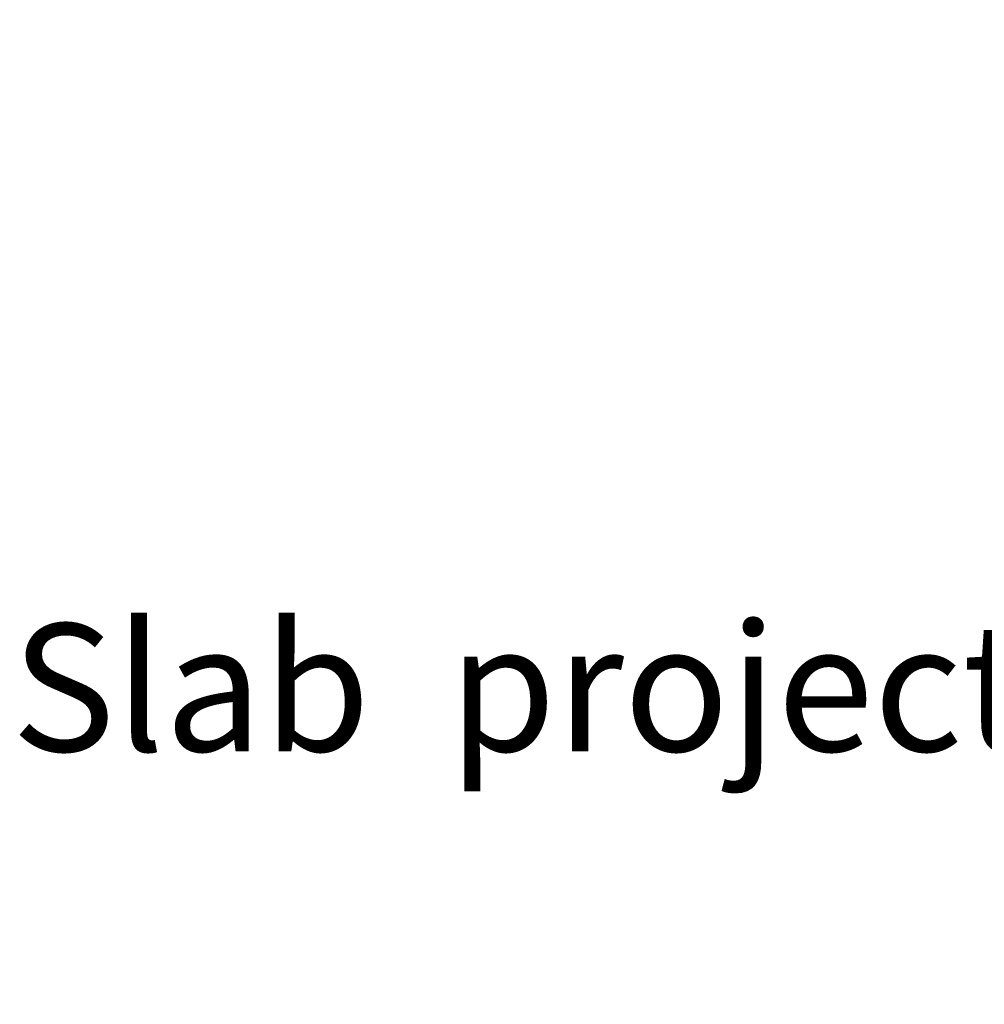
# Model space of a CAD drawing. Units: metres. Extents: x 5.2 to 41.7, y 12.2 to 37.4.
# Tile 1 of 6: x 18.078 to 19.439, y 14.432 to 15.821. Entities that reach past the tile are written whole.
import ezdxf
from ezdxf import colors
from ezdxf.entities.mleader import LeaderData, LeaderLine
from ezdxf.math import Vec2, Vec3

# ---------------------------------------------------------------- set-up
doc = ezdxf.new("R2010")
doc.units = ezdxf.units.M
doc.header["$MEASUREMENT"] = 0
doc.layers.add('A-ANNO-TEXT', color=3, linetype='Continuous', lineweight=18)
doc.styles.get("Standard").update_dxf_attribs({"font": 'arial.ttf'})

msp = doc.modelspace()

# ---------------------------------------------------------------- leaders
at = {"layer": 'A-ANNO-TEXT'}
ml = msp.add_multileader_mtext('Standard', dxfattribs=at)
ml.set_content('Slab  projection ', color=256)
ml.set_leader_properties()
ml.build(insert=Vec2(0, 0))
ml.multileader.update_dxf_attribs({"dogleg_length": 0.36, "arrow_head_size": 0.18})
ctx = ml.context
ctx.base_point, ctx.char_height, ctx.arrow_head_size, ctx.landing_gap_size, ctx.plane_origin = Vec3(18.07181, 14.85251), 0.18, 0.18, 0.09, Vec3(20.72542, 15.63365)
ctx.text_align_type = 2
notes = []
notes.append((ctx, [(1, (1, 1, 0), (20.8335, 14.85251), (-1, 0), 0.87697, [(0, [(20.93558, 15.82081)], 0, [])])]))
ctx.mtext.insert, ctx.mtext.alignment, ctx.mtext.flow_direction = Vec3(19.86653, 14.96897), 3, 5
for ctx, leaders in notes:
    for number, flags, end, landing, length, lines in leaders:
        leader = LeaderData()
        leader.index, (leader.has_last_leader_line, leader.has_dogleg_vector, leader.attachment_direction) = number, flags
        leader.last_leader_point, leader.dogleg_vector, leader.dogleg_length = Vec3(end), Vec3(landing), length
        for number, points, colour, breaks in lines:
            line = LeaderLine()
            line.index, line.vertices, line.color, line.breaks = number, Vec3.list(points), colors.encode_raw_color(colour), breaks
            leader.lines.append(line)
        ctx.leaders.append(leader)

doc.saveas('drawing.dxf')
